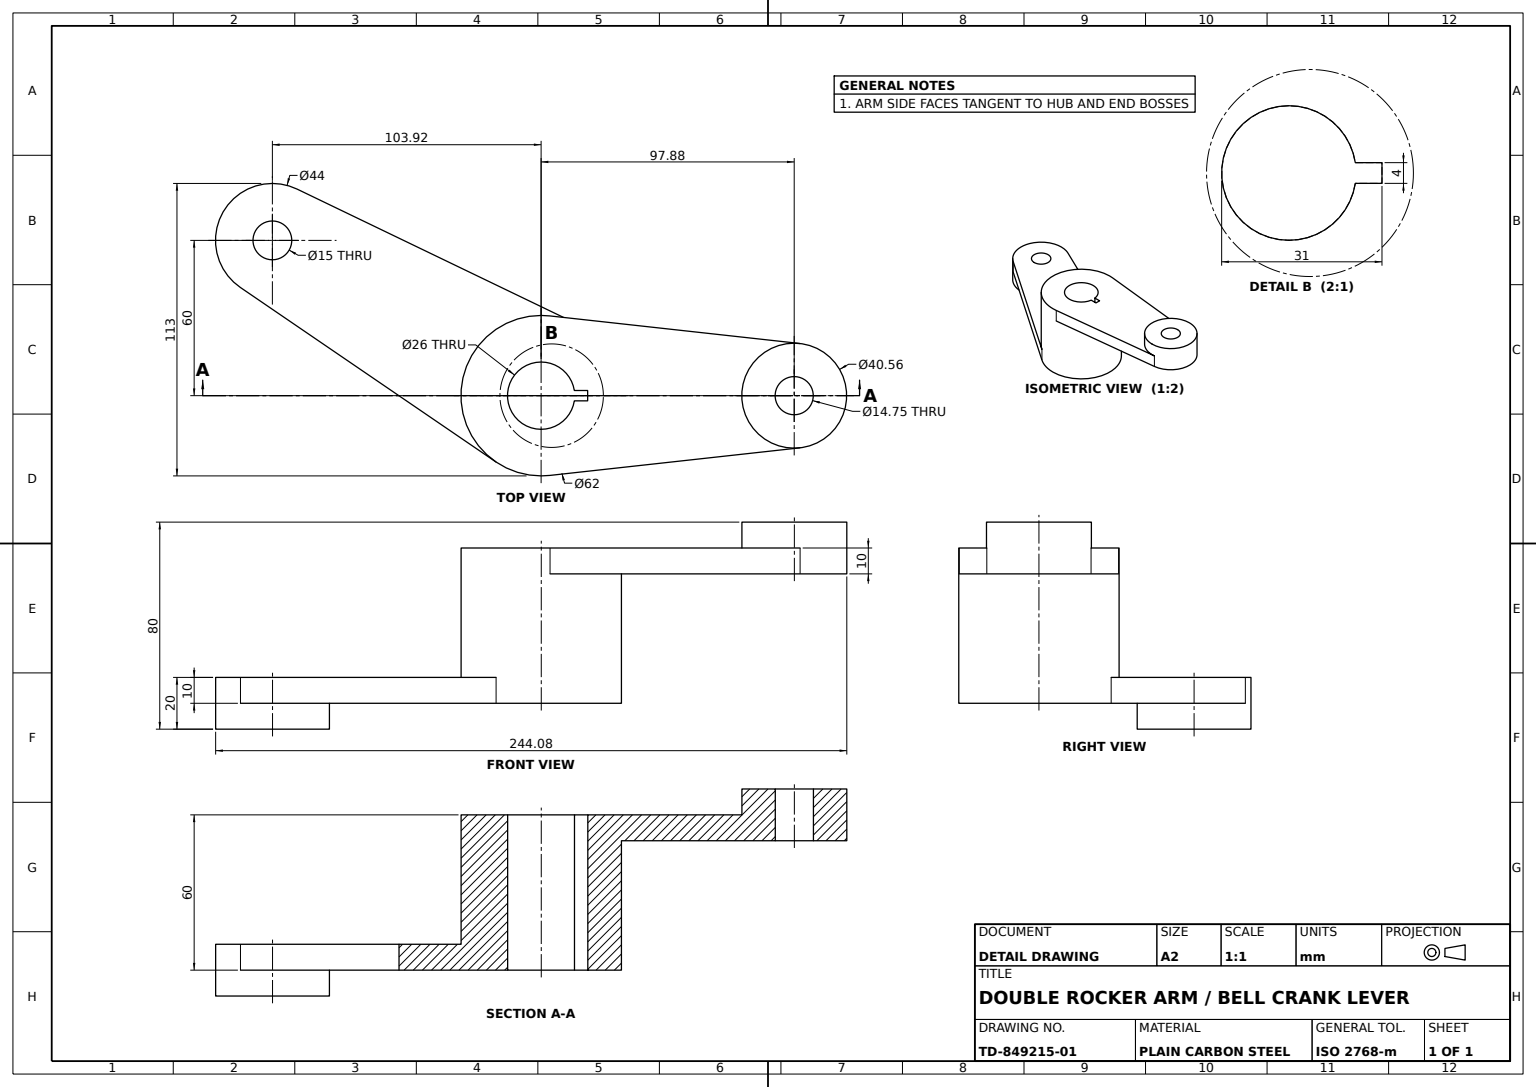
from build123d import *

# Parameters (mm, degrees)
HUB_PROFILE_SKETCH_R       = 31
HUB_62_KEYED_BORE_26_DEPTH = 50
ARM_A_PLATE_DEPTH          = 10
SKETCH2_4_R                = 20.281835497
SKETCH2_4_R_2              = 7.37420564
ARM_A_END_BOSS_DEPTH       = 20
ARM_B_PLATE_DEPTH          = 10
ARM_B_END_BOSS_DEPTH       = 10
ARM_B_END_BOSS_DEPTH_BACK  = 10
SKETCH4_3_R                = 22
SKETCH4_3_R_2              = 7.5


with BuildPart() as part:
    # Hub Profile Sketch → Hub _62 Keyed Bore _26 (new body)
    with BuildSketch(Plane(origin=(0, 0, 0), x_dir=(1, 0, 0), z_dir=(0, 1, 0))):
        with Locations(Location((0, 0, 0), (0, 0, 270))):
            Circle(HUB_PROFILE_SKETCH_R)
        with BuildLine():
            Line((12.845232579, -2), (18, -2))
            Line((18, -2), (18, 2))
            Line((18, 2), (12.845232579, 2))
            ThreePointArc((12.845232579, 2), (-13, 0), (12.845232579, -2))
        make_face(mode=Mode.SUBTRACT)
    extrude(amount=HUB_62_KEYED_BORE_26_DEPTH)

    # Arm A Sketch → Arm A Plate (add)
    with BuildSketch(Plane(origin=(0, 50, 0), x_dir=(1, 0, 0), z_dir=(0, 1, 0))):
        with BuildLine():
            ThreePointArc((3.394741403, 30.813564072), (-31, 0), (3.394741403, -30.813564072))
            Line((3.394741403, -30.813564072), (100.096839243, -20.159859277))
            ThreePointArc((100.096839243, -20.159859277), (77.593984821, 0), (100.096839243, 20.159859277))
            Line((100.096839243, 20.159859277), (3.394741403, 30.813564072))
        make_face()
        with BuildLine():
            Line((18, 2), (18, 0))
            Line((18, 0), (18, -2))
            Line((18, -2), (12.845232579, -2))
            ThreePointArc((12.845232579, -2), (-13, 0), (12.845232579, 2))
            Line((12.845232579, 2), (18, 2))
        make_face(mode=Mode.SUBTRACT)
    extrude(amount=ARM_A_PLATE_DEPTH)

    # Sketch2_4 → Arm A End Boss (add)
    with BuildSketch(Plane(origin=(0, 50, 0), x_dir=(1, 0, 0), z_dir=(0, 1, 0))):
        with Locations(Location((97.875820318, 0, 0), (0, 0, 83.713057555))):
            Circle(SKETCH2_4_R)
        with Locations(Location((97.875820318, 0, 0), (0, 0, 270))):
            Circle(SKETCH2_4_R_2, mode=Mode.SUBTRACT)
    extrude(amount=ARM_A_END_BOSS_DEPTH)

    # Arm B Sketch → Arm B Plate (add)
    with BuildSketch(Plane.XZ):
        with BuildLine():
            Line((-17.469853837, 25.608674447), (-116.321009242, -41.826102006))
            ThreePointArc((-116.321009242, -41.826102006), (-93.645771026, -40.54807031), (-81.923048454, -60))
            ThreePointArc((-81.923048454, -60), (-85.296700275, -71.70722655), (-94.382971499, -79.823897994))
            Line((-94.382971499, -79.823897994), (13.442835709, -27.933674447))
            ThreePointArc((13.442835709, -27.933674447), (-26.846787517, -15.5), (-17.469853837, 25.608674447))
        make_face()
    extrude(amount=-ARM_B_PLATE_DEPTH)

    # Sketch4_3 → Arm B End Boss (add, two sides: drawn at the far end of the back side and taken through both)
    with BuildSketch(Plane.XZ.offset(-ARM_B_END_BOSS_DEPTH_BACK)):
        with Locations(Location((-103.923048454, -60, 0), (0, 0, 124.301222305))):
            Circle(SKETCH4_3_R)
        with Locations(Location((-103.923048454, -60, 0), (0, 0, 270))):
            Circle(SKETCH4_3_R_2, mode=Mode.SUBTRACT)
    extrude(amount=ARM_B_END_BOSS_DEPTH + ARM_B_END_BOSS_DEPTH_BACK)


solid = part.part
